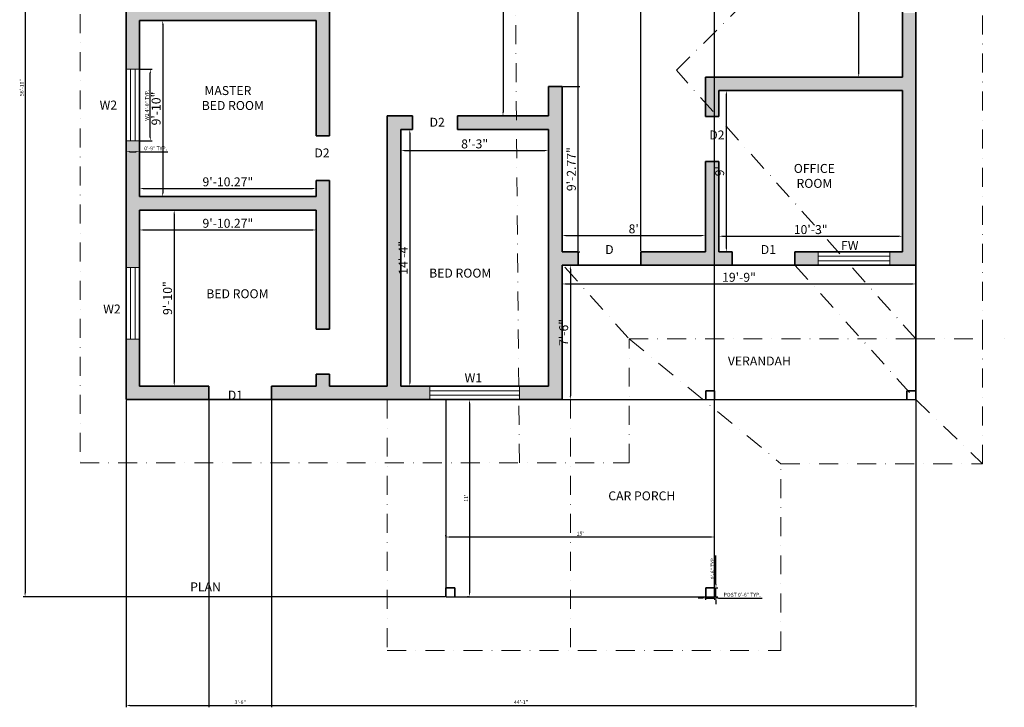
# Model space of a CAD drawing. Units: inches. Extents: x 4701 to 5398, y 2331 to 3130.
# Tile 1 of 3: x 4701 to 5360, y 2331 to 2792. Entities that reach past the tile are written whole.
import ezdxf

# ---------------------------------------------------------------- set-up
doc = ezdxf.new("R2010")
doc.units = ezdxf.units.IN
doc.linetypes.add('DASHDOT', pattern=[25.4, 12.7, -6.35, 0, -6.35])
for name, color, linetype, lineweight, true_color in [('A-ANNO-DIMS', 217, 'Continuous', 18, 0x93278f), ('A-GLAZ', 41, 'Continuous', 18, 0xf4ee51), ('A-WALL-PATT', 143, 'Continuous', 13, 0x7aafdf)]:
    doc.layers.add(name, color=color, linetype=linetype, lineweight=lineweight, true_color=true_color)
for name, color, linetype, lineweight in [('A-ANNO-TEXT', 7, 'Continuous', 18), ('A-AREA-IDEN', 7, 'Continuous', 25), ('A-COLS', 7, 'Continuous', 35), ('A-FLOR-OTLN', 7, 'Continuous', 25), ('A-ROOF-OVHD', 8, 'DASHDOT', 13), ('A-WALL', 7, 'Continuous', 35)]:
    doc.layers.add(name, color=color, linetype=linetype, lineweight=lineweight)
doc.styles.get("Standard").update_dxf_attribs({"font": 'arial.ttf'})
doc.dimstyles.new('ISO-25', dxfattribs={"dimtxt": 2.5, "dimasz": 2.5, "dimexe": 1.25, "dimexo": 0.625, "dimtad": 1, "dimlunit": 3, "dimtxsty": 'Standard', "dimcen": 2.5, "dimadec": 0, "dimazin": 0, "dimtfac": 1, "dimtmove": 0, "dimatfit": 3, "dimfxl": 1, "dimarcsym": 0})

# ---------------------------------------------------------------- blocks, each defined once
blk = doc.blocks.new('*D12')
at = {"layer": 'A-ANNO-DIMS', "color": 0, "lineweight": -2, "transparency": 16777216}
for p, q in [((5262.75, 2882.55), (5262.75, 2755.55)), ((5263.38, 2885.05), (5264, 2885.05)), ((5263.38, 2753.05), (5264, 2753.05))]:
    blk.add_line(p, q, dxfattribs=at)
at = {"layer": 'A-ANNO-DIMS', "color": 0, "transparency": 16777216}
for points in [[(5262.34, 2882.55), (5263.17, 2882.55), (5262.75, 2885.05)], [(5262.34, 2755.55), (5263.17, 2755.55), (5262.75, 2753.05)]]:
    blk.add_solid(points, dxfattribs=at)
at = {"layer": 'Defpoints', "color": 0, "transparency": 16777216}
for p in [(5262.75, 2885.05), (5262.75, 2753.05), (5262.75, 2753.05)]:
    blk.add_point(p, dxfattribs=at)
at = {"layer": 'A-ANNO-DIMS', "color": 0, "transparency": 16777216, "insert": (5259.12, 2819.05), "char_height": 6, "attachment_point": 5, "rotation": 90}
blk.add_mtext("11'", dxfattribs=at)
blk = doc.blocks.new('*D15')
at = {"layer": 'A-ANNO-DIMS', "color": 0, "lineweight": -2, "transparency": 16777216}
for p, q in [((4797.37, 2791.05), (4798, 2791.05)), ((4796.75, 2788.55), (4796.75, 2675.55)), ((4797.37, 2673.05), (4798, 2673.05))]:
    blk.add_line(p, q, dxfattribs=at)
at = {"layer": 'A-ANNO-DIMS', "color": 0, "transparency": 16777216}
for points in [[(4796.33, 2788.55), (4797.17, 2788.55), (4796.75, 2791.05)], [(4796.33, 2675.55), (4797.17, 2675.55), (4796.75, 2673.05)]]:
    blk.add_solid(points, dxfattribs=at)
at = {"layer": 'Defpoints', "color": 0, "transparency": 16777216}
for p in [(4796.75, 2791.05), (4796.75, 2673.05), (4796.75, 2673.05)]:
    blk.add_point(p, dxfattribs=at)
at = {"layer": 'A-ANNO-DIMS', "color": 0, "transparency": 16777216, "insert": (4793.06, 2732.05), "char_height": 6, "attachment_point": 5, "rotation": 90}
blk.add_mtext('9\'-10"', dxfattribs=at)
blk = doc.blocks.new('*D16')
at = {"layer": 'A-ANNO-DIMS', "color": 0, "lineweight": -2, "transparency": 16777216}
for p, q in [((4781.22, 2679.07), (4781.22, 2679.7)), ((4783.72, 2678.45), (4897, 2678.45)), ((4899.5, 2679.07), (4899.5, 2679.7))]:
    blk.add_line(p, q, dxfattribs=at)
at = {"layer": 'A-ANNO-DIMS', "color": 0, "transparency": 16777216}
for points in [[(4783.72, 2678.87), (4783.72, 2678.03), (4781.22, 2678.45)], [(4897, 2678.87), (4897, 2678.03), (4899.5, 2678.45)]]:
    blk.add_solid(points, dxfattribs=at)
at = {"layer": 'Defpoints', "color": 0, "transparency": 16777216}
for p in [(4781.22, 2678.45), (4899.5, 2678.45), (4899.5, 2678.45)]:
    blk.add_point(p, dxfattribs=at)
at = {"layer": 'A-ANNO-DIMS', "color": 0, "transparency": 16777216, "insert": (4840.36, 2682.14), "char_height": 6, "attachment_point": 5}
blk.add_mtext('9\'-10.27"', dxfattribs=at)
blk = doc.blocks.new('*D17')
at = {"layer": 'A-ANNO-DIMS', "color": 0, "lineweight": -2, "transparency": 16777216}
for p, q in [((4805.06, 2664.05), (4805.69, 2664.05)), ((4804.44, 2661.55), (4804.44, 2548.55)), ((4805.06, 2546.05), (4805.69, 2546.05))]:
    blk.add_line(p, q, dxfattribs=at)
at = {"layer": 'A-ANNO-DIMS', "color": 0, "transparency": 16777216}
for points in [[(4804.02, 2661.55), (4804.86, 2661.55), (4804.44, 2664.05)], [(4804.02, 2548.55), (4804.86, 2548.55), (4804.44, 2546.05)]]:
    blk.add_solid(points, dxfattribs=at)
at = {"layer": 'Defpoints', "color": 0, "transparency": 16777216}
for p in [(4804.44, 2664.05), (4804.44, 2546.05), (4804.44, 2546.05)]:
    blk.add_point(p, dxfattribs=at)
at = {"layer": 'A-ANNO-DIMS', "color": 0, "transparency": 16777216, "insert": (4800.75, 2605.05), "char_height": 6, "attachment_point": 5, "rotation": 90}
blk.add_mtext('9\'-10"', dxfattribs=at)
blk = doc.blocks.new('*D18')
at = {"layer": 'A-ANNO-DIMS', "color": 0, "lineweight": -2, "transparency": 16777216}
for p, q in [((4781.22, 2651.33), (4781.22, 2651.95)), ((4783.72, 2650.7), (4897, 2650.7)), ((4899.5, 2651.33), (4899.5, 2651.95))]:
    blk.add_line(p, q, dxfattribs=at)
at = {"layer": 'A-ANNO-DIMS', "color": 0, "transparency": 16777216}
for points in [[(4783.72, 2651.12), (4783.72, 2650.29), (4781.22, 2650.7)], [(4897, 2651.12), (4897, 2650.29), (4899.5, 2650.7)]]:
    blk.add_solid(points, dxfattribs=at)
at = {"layer": 'Defpoints', "color": 0, "transparency": 16777216}
for p in [(4781.22, 2650.7), (4899.5, 2650.7), (4899.5, 2650.7)]:
    blk.add_point(p, dxfattribs=at)
at = {"layer": 'A-ANNO-DIMS', "color": 0, "transparency": 16777216, "insert": (4840.36, 2654.39), "char_height": 6, "attachment_point": 5}
blk.add_mtext('9\'-10.27"', dxfattribs=at)
blk = doc.blocks.new('*D19')
at = {"layer": 'A-ANNO-DIMS', "color": 0, "lineweight": -2, "transparency": 16777216}
for p, q in [((4961.57, 2718.05), (4960.94, 2718.05)), ((4962.19, 2715.55), (4962.19, 2548.55)), ((4961.57, 2546.05), (4960.94, 2546.05))]:
    blk.add_line(p, q, dxfattribs=at)
at = {"layer": 'A-ANNO-DIMS', "color": 0, "transparency": 16777216}
for points in [[(4961.78, 2715.55), (4962.61, 2715.55), (4962.19, 2718.05)], [(4961.78, 2548.55), (4962.61, 2548.55), (4962.19, 2546.05)]]:
    blk.add_solid(points, dxfattribs=at)
at = {"layer": 'Defpoints', "color": 0, "transparency": 16777216}
for p in [(4962.19, 2718.05), (4962.19, 2546.05), (4962.19, 2546.05)]:
    blk.add_point(p, dxfattribs=at)
at = {"layer": 'A-ANNO-DIMS', "color": 0, "transparency": 16777216, "insert": (4958.56, 2632.05), "char_height": 6, "attachment_point": 5, "rotation": 90}
blk.add_mtext('14\'-4"', dxfattribs=at)
blk = doc.blocks.new('*D20')
at = {"layer": 'A-ANNO-DIMS', "color": 0, "lineweight": -2, "transparency": 16777216}
for p, q in [((4956.11, 2704.5), (4956.11, 2705.12)), ((4958.61, 2703.87), (5052.61, 2703.87)), ((5055.11, 2704.5), (5055.11, 2705.12))]:
    blk.add_line(p, q, dxfattribs=at)
at = {"layer": 'A-ANNO-DIMS', "color": 0, "transparency": 16777216}
for points in [[(4958.61, 2704.29), (4958.61, 2703.46), (4956.11, 2703.87)], [(5052.61, 2704.29), (5052.61, 2703.46), (5055.11, 2703.87)]]:
    blk.add_solid(points, dxfattribs=at)
at = {"layer": 'Defpoints', "color": 0, "transparency": 16777216}
for p in [(4956.11, 2703.87), (5055.11, 2703.87), (5055.11, 2703.87)]:
    blk.add_point(p, dxfattribs=at)
at = {"layer": 'A-ANNO-DIMS', "color": 0, "transparency": 16777216, "insert": (5005.61, 2707.56), "char_height": 6, "attachment_point": 5}
blk.add_mtext('8\'-3"', dxfattribs=at)
blk = doc.blocks.new('*D21')
at = {"layer": 'A-ANNO-DIMS', "color": 0, "lineweight": -2, "transparency": 16777216}
for p, q in [((5001.51, 2537.05), (5000.88, 2537.05)), ((5002.13, 2534.55), (5002.13, 2407.55)), ((5001.51, 2405.05), (5000.88, 2405.05))]:
    blk.add_line(p, q, dxfattribs=at)
at = {"layer": 'A-ANNO-DIMS', "color": 0, "transparency": 16777216}
for points in [[(5001.72, 2534.55), (5002.55, 2534.55), (5002.13, 2537.05)], [(5001.72, 2407.55), (5002.55, 2407.55), (5002.13, 2405.05)]]:
    blk.add_solid(points, dxfattribs=at)
at = {"layer": 'Defpoints', "color": 0, "transparency": 16777216}
for p in [(5002.13, 2537.05), (5002.13, 2405.05), (5002.13, 2405.05)]:
    blk.add_point(p, dxfattribs=at)
at = {"layer": 'A-ANNO-DIMS', "color": 0, "transparency": 16777216, "insert": (5000.25, 2471.05), "char_height": 2.5, "attachment_point": 5, "rotation": 90}
blk.add_mtext("11'", dxfattribs=at)
blk = doc.blocks.new('*D22')
at = {"layer": 'A-ANNO-DIMS', "color": 0, "lineweight": -2, "transparency": 16777216}
for p, q in [((4986.3, 2445.66), (4986.3, 2446.29)), ((5166.3, 2445.66), (5166.3, 2446.29)), ((4988.8, 2445.04), (5163.8, 2445.04))]:
    blk.add_line(p, q, dxfattribs=at)
at = {"layer": 'A-ANNO-DIMS', "color": 0, "transparency": 16777216}
for points in [[(4988.8, 2445.45), (4988.8, 2444.62), (4986.3, 2445.04)], [(5163.8, 2445.45), (5163.8, 2444.62), (5166.3, 2445.04)]]:
    blk.add_solid(points, dxfattribs=at)
at = {"layer": 'Defpoints', "color": 0, "transparency": 16777216}
for p in [(4986.3, 2445.04), (5166.3, 2445.04), (5166.3, 2445.04)]:
    blk.add_point(p, dxfattribs=at)
at = {"layer": 'A-ANNO-DIMS', "color": 0, "transparency": 16777216, "insert": (5076.3, 2446.94), "char_height": 2.5, "attachment_point": 5}
blk.add_mtext("15'", dxfattribs=at)
blk = doc.blocks.new('*D23')
at = {"layer": 'A-ANNO-DIMS', "color": 0, "lineweight": -2, "transparency": 16777216}
for p, q in [((5064.11, 2615.15), (5064.11, 2615.78)), ((5066.61, 2614.53), (5298.61, 2614.53)), ((5301.11, 2615.15), (5301.11, 2615.78))]:
    blk.add_line(p, q, dxfattribs=at)
at = {"layer": 'A-ANNO-DIMS', "color": 0, "transparency": 16777216}
for points in [[(5066.61, 2614.94), (5066.61, 2614.11), (5064.11, 2614.53)], [(5298.61, 2614.94), (5298.61, 2614.11), (5301.11, 2614.53)]]:
    blk.add_solid(points, dxfattribs=at)
at = {"layer": 'Defpoints', "color": 0, "transparency": 16777216}
for p in [(5064.11, 2614.53), (5301.11, 2614.53), (5301.11, 2614.53)]:
    blk.add_point(p, dxfattribs=at)
at = {"layer": 'A-ANNO-DIMS', "color": 0, "transparency": 16777216, "insert": (5182.61, 2618.22), "char_height": 6, "attachment_point": 5}
blk.add_mtext('19\'-9"', dxfattribs=at)
blk = doc.blocks.new('*D24')
at = {"layer": 'A-ANNO-DIMS', "color": 0, "lineweight": -2, "transparency": 16777216}
for p, q in [((5069.69, 2624.55), (5069.69, 2539.55)), ((5070.31, 2627.05), (5070.94, 2627.05)), ((5070.31, 2537.05), (5070.94, 2537.05))]:
    blk.add_line(p, q, dxfattribs=at)
at = {"layer": 'A-ANNO-DIMS', "color": 0, "transparency": 16777216}
for points in [[(5069.27, 2624.55), (5070.1, 2624.55), (5069.69, 2627.05)], [(5069.27, 2539.55), (5070.1, 2539.55), (5069.69, 2537.05)]]:
    blk.add_solid(points, dxfattribs=at)
at = {"layer": 'Defpoints', "color": 0, "transparency": 16777216}
for p in [(5069.69, 2627.05), (5069.69, 2537.05), (5069.69, 2537.05)]:
    blk.add_point(p, dxfattribs=at)
at = {"layer": 'A-ANNO-DIMS', "color": 0, "transparency": 16777216, "insert": (5066, 2582.05), "char_height": 6, "attachment_point": 5, "rotation": 90}
blk.add_mtext('7\'-6"', dxfattribs=at)
blk = doc.blocks.new('*D25')
at = {"layer": 'A-ANNO-DIMS', "color": 0, "lineweight": -2, "transparency": 16777216}
for p, q in [((5064.11, 2647.58), (5064.11, 2648.21)), ((5066.61, 2646.96), (5157.61, 2646.96)), ((5160.11, 2647.58), (5160.11, 2648.21))]:
    blk.add_line(p, q, dxfattribs=at)
at = {"layer": 'A-ANNO-DIMS', "color": 0, "transparency": 16777216}
for points in [[(5066.61, 2647.38), (5066.61, 2646.54), (5064.11, 2646.96)], [(5157.61, 2647.38), (5157.61, 2646.54), (5160.11, 2646.96)]]:
    blk.add_solid(points, dxfattribs=at)
at = {"layer": 'Defpoints', "color": 0, "transparency": 16777216}
for p in [(5064.11, 2646.96), (5160.11, 2646.96), (5160.11, 2646.96)]:
    blk.add_point(p, dxfattribs=at)
at = {"layer": 'A-ANNO-DIMS', "color": 0, "transparency": 16777216, "insert": (5112.11, 2650.65), "char_height": 6, "attachment_point": 5}
blk.add_mtext("8'", dxfattribs=at)
blk = doc.blocks.new('*D26')
at = {"layer": 'A-ANNO-DIMS', "color": 0, "lineweight": -2, "transparency": 16777216}
for p, q in [((5064.73, 2746.83), (5076.07, 2746.83)), ((5074.82, 2638.55), (5074.82, 2744.33)), ((5070.84, 2636.05), (5076.07, 2636.05))]:
    blk.add_line(p, q, dxfattribs=at)
at = {"layer": 'A-ANNO-DIMS', "color": 0, "transparency": 16777216}
for points in [[(5074.4, 2744.33), (5075.24, 2744.33), (5074.82, 2746.83)], [(5074.4, 2638.55), (5075.24, 2638.55), (5074.82, 2636.05)]]:
    blk.add_solid(points, dxfattribs=at)
at = {"layer": 'Defpoints', "color": 0, "transparency": 16777216}
for p in [(5064.11, 2746.83), (5074.82, 2746.83), (5070.21, 2636.05)]:
    blk.add_point(p, dxfattribs=at)
at = {"layer": 'A-ANNO-DIMS', "color": 0, "transparency": 16777216, "insert": (5071.13, 2691.44), "char_height": 6, "attachment_point": 5, "rotation": 90}
blk.add_mtext('9\'-2.77"', dxfattribs=at)
blk = doc.blocks.new('*D27')
at = {"layer": 'A-ANNO-DIMS', "color": 0, "lineweight": -2, "transparency": 16777216}
for p, q in [((5169.11, 2647.11), (5169.11, 2647.74)), ((5171.61, 2646.49), (5289.61, 2646.49)), ((5292.11, 2647.11), (5292.11, 2647.74))]:
    blk.add_line(p, q, dxfattribs=at)
at = {"layer": 'A-ANNO-DIMS', "color": 0, "transparency": 16777216}
for points in [[(5171.61, 2646.9), (5171.61, 2646.07), (5169.11, 2646.49)], [(5289.61, 2646.9), (5289.61, 2646.07), (5292.11, 2646.49)]]:
    blk.add_solid(points, dxfattribs=at)
at = {"layer": 'Defpoints', "color": 0, "transparency": 16777216}
for p in [(5169.11, 2646.49), (5292.11, 2646.49), (5292.11, 2646.49)]:
    blk.add_point(p, dxfattribs=at)
at = {"layer": 'A-ANNO-DIMS', "color": 0, "transparency": 16777216, "insert": (5230.61, 2650.18), "char_height": 6, "attachment_point": 5}
blk.add_mtext('10\'-3"', dxfattribs=at)
blk = doc.blocks.new('*D28')
at = {"layer": 'A-ANNO-DIMS', "color": 0, "lineweight": -2, "transparency": 16777216}
for p, q in [((5174.78, 2744.05), (5175.4, 2744.05)), ((5174.15, 2638.55), (5174.15, 2741.55)), ((5174.78, 2636.05), (5175.4, 2636.05))]:
    blk.add_line(p, q, dxfattribs=at)
at = {"layer": 'A-ANNO-DIMS', "color": 0, "transparency": 16777216}
for points in [[(5173.74, 2741.55), (5174.57, 2741.55), (5174.15, 2744.05)], [(5173.74, 2638.55), (5174.57, 2638.55), (5174.15, 2636.05)]]:
    blk.add_solid(points, dxfattribs=at)
at = {"layer": 'Defpoints', "color": 0, "transparency": 16777216}
for p in [(5174.15, 2744.05), (5174.15, 2744.05), (5174.15, 2636.05)]:
    blk.add_point(p, dxfattribs=at)
at = {"layer": 'A-ANNO-DIMS', "color": 0, "transparency": 16777216, "insert": (5170.46, 2690.05), "char_height": 6, "attachment_point": 5, "rotation": 90}
blk.add_mtext("9'", dxfattribs=at)
blk = doc.blocks.new('*D30')
at = {"layer": 'A-ANNO-DIMS', "color": 0, "lineweight": -2, "transparency": 16777216}
for p, q in [((5024.48, 2894.05), (5023.35, 2894.05)), ((5024.6, 2891.55), (5024.6, 2729.55)), ((5025.23, 2727.05), (5025.85, 2727.05))]:
    blk.add_line(p, q, dxfattribs=at)
at = {"layer": 'A-ANNO-DIMS', "color": 0, "transparency": 16777216}
for points in [[(5024.19, 2891.55), (5025.02, 2891.55), (5024.6, 2894.05)], [(5024.19, 2729.55), (5025.02, 2729.55), (5024.6, 2727.05)]]:
    blk.add_solid(points, dxfattribs=at)
at = {"layer": 'Defpoints', "color": 0, "transparency": 16777216}
for p in [(5025.11, 2894.05), (5024.6, 2727.05), (5024.6, 2727.05)]:
    blk.add_point(p, dxfattribs=at)
at = {"layer": 'A-ANNO-DIMS', "color": 0, "transparency": 16777216, "insert": (5022.7, 2810.55), "char_height": 2.5, "attachment_point": 5, "rotation": 90}
blk.add_mtext('13\'-11"', dxfattribs=at)
blk = doc.blocks.new('WIN-48IN')
for p, q in [((0, 48), (9, 48)), ((0, 48), (0, 0)), ((3, 48), (3, 0)), ((6, 48), (6, 0)), ((9, 0), (9, 48)), ((0, 0), (9, 0))]:
    blk.add_line(p, q)
blk = doc.blocks.new('WIN-60IN')
for p, q in [((0, 9), (0, 0)), ((0, 9), (60, 9)), ((60, 9), (60, 0)), ((0, 6), (60, 6)), ((0, 3), (60, 3)), ((60, 0), (0, 0))]:
    blk.add_line(p, q)
blk = doc.blocks.new('POST-6X6IN')
for p, q in [((0, 0), (0, 6)), ((0, 6), (6, 6)), ((6, 6), (6, 0))]:
    blk.add_line(p, q)
blk = doc.blocks.new('*D35')
at = {"layer": 'A-ANNO-DIMS', "color": 0, "lineweight": -2, "transparency": 16777216}
for p, q in [((4781.85, 2758.33), (4789.67, 2758.33)), ((4788.42, 2712.83), (4788.42, 2755.83)), ((4781.85, 2710.33), (4789.67, 2710.33))]:
    blk.add_line(p, q, dxfattribs=at)
at = {"layer": 'A-ANNO-DIMS', "color": 0, "transparency": 16777216}
for points in [[(4788.01, 2755.83), (4788.84, 2755.83), (4788.42, 2758.33)], [(4788.01, 2712.83), (4788.84, 2712.83), (4788.42, 2710.33)]]:
    blk.add_solid(points, dxfattribs=at)
at = {"layer": 'Defpoints', "color": 0, "transparency": 16777216}
for p in [(4781.22, 2758.33), (4788.42, 2758.33), (4781.22, 2710.33)]:
    blk.add_point(p, dxfattribs=at)
at = {"layer": 'A-ANNO-DIMS', "color": 0, "transparency": 16777216, "insert": (4786.52, 2734.33), "char_height": 2.5, "attachment_point": 5, "rotation": 90}
blk.add_mtext('W2 4\'-0" TYP.', dxfattribs=at)
blk = doc.blocks.new('*D36')
at = {"layer": 'A-ANNO-DIMS', "color": 0, "lineweight": -2, "transparency": 16777216}
for p, q in [((4772.22, 2709.71), (4772.22, 2701.88)), ((4781.22, 2709.71), (4781.22, 2701.88)), ((4774.72, 2703.13), (4778.72, 2703.13)), ((4781.22, 2703.13), (4800.21, 2703.13))]:
    blk.add_line(p, q, dxfattribs=at)
at = {"layer": 'A-ANNO-DIMS', "color": 0, "transparency": 16777216}
for points in [[(4774.72, 2703.55), (4774.72, 2702.72), (4772.22, 2703.13)], [(4778.72, 2703.55), (4778.72, 2702.72), (4781.22, 2703.13)]]:
    blk.add_solid(points, dxfattribs=at)
at = {"layer": 'Defpoints', "color": 0, "transparency": 16777216}
for p in [(4772.22, 2710.33), (4781.22, 2710.33), (4781.22, 2703.13)]:
    blk.add_point(p, dxfattribs=at)
at = {"layer": 'A-ANNO-DIMS', "color": 0, "transparency": 16777216, "insert": (4791.97, 2705.04), "char_height": 2.5, "attachment_point": 5}
blk.add_mtext('0\'-9" TYP.', dxfattribs=at)
blk = doc.blocks.new('*D41')
at = {"layer": 'A-ANNO-DIMS', "color": 0, "lineweight": -2, "transparency": 16777216}
for p, q in [((5157.8, 2404.15), (5155.3, 2404.15)), ((5160.3, 2404.43), (5160.3, 2402.9)), ((5160.3, 2404.15), (5166.3, 2404.15)), ((5166.3, 2404.43), (5166.3, 2402.9)), ((5168.8, 2404.15), (5198.15, 2404.15))]:
    blk.add_line(p, q, dxfattribs=at)
at = {"layer": 'A-ANNO-DIMS', "color": 0, "transparency": 16777216}
for points in [[(5157.8, 2404.57), (5157.8, 2403.74), (5160.3, 2404.15)], [(5168.8, 2404.57), (5168.8, 2403.74), (5166.3, 2404.15)]]:
    blk.add_solid(points, dxfattribs=at)
at = {"layer": 'Defpoints', "color": 0, "transparency": 16777216}
for p in [(5160.3, 2405.05), (5166.3, 2405.05), (5166.3, 2404.15)]:
    blk.add_point(p, dxfattribs=at)
at = {"layer": 'A-ANNO-DIMS', "color": 0, "transparency": 16777216, "insert": (5184.73, 2406.07), "char_height": 2.5, "attachment_point": 5}
blk.add_mtext('POST 0\'-6" TYP.', dxfattribs=at)
blk = doc.blocks.new('*D42')
at = {"layer": 'A-ANNO-DIMS', "color": 0, "lineweight": -2, "transparency": 16777216}
for p, q in [((5167.2, 2413.55), (5167.2, 2432.54)), ((5166.93, 2411.05), (5168.45, 2411.05)), ((5167.2, 2405.05), (5167.2, 2411.05)), ((5166.93, 2405.05), (5168.45, 2405.05)), ((5167.2, 2402.55), (5167.2, 2400.05))]:
    blk.add_line(p, q, dxfattribs=at)
at = {"layer": 'A-ANNO-DIMS', "color": 0, "transparency": 16777216}
for points in [[(5166.79, 2413.55), (5167.62, 2413.55), (5167.2, 2411.05)], [(5166.79, 2402.55), (5167.62, 2402.55), (5167.2, 2405.05)]]:
    blk.add_solid(points, dxfattribs=at)
at = {"layer": 'Defpoints', "color": 0, "transparency": 16777216}
for p in [(5166.3, 2411.05), (5167.2, 2411.05), (5166.3, 2405.05)]:
    blk.add_point(p, dxfattribs=at)
at = {"layer": 'A-ANNO-DIMS', "color": 0, "transparency": 16777216, "insert": (5165.3, 2424.3), "char_height": 2.5, "attachment_point": 5, "rotation": 90}
blk.add_mtext('0\'-6" TYP.', dxfattribs=at)
blk = doc.blocks.new('*D43')
at = {"layer": 'A-ANNO-DIMS', "color": 0, "lineweight": -2, "transparency": 16777216}
for p, q in [((4772.22, 2536.43), (4772.22, 2330.95)), ((5301.11, 2536.43), (5301.11, 2330.95)), ((4774.72, 2332.2), (5298.61, 2332.2))]:
    blk.add_line(p, q, dxfattribs=at)
at = {"layer": 'A-ANNO-DIMS', "color": 0, "transparency": 16777216}
for points in [[(4774.72, 2332.62), (4774.72, 2331.79), (4772.22, 2332.2)], [(5298.61, 2332.62), (5298.61, 2331.79), (5301.11, 2332.2)]]:
    blk.add_solid(points, dxfattribs=at)
at = {"layer": 'Defpoints', "color": 0, "transparency": 16777216}
for p in [(4772.22, 2537.05), (5301.11, 2537.05), (5301.11, 2332.2)]:
    blk.add_point(p, dxfattribs=at)
at = {"layer": 'A-ANNO-DIMS', "color": 0, "transparency": 16777216, "insert": (5036.67, 2334.08), "char_height": 2.5, "attachment_point": 5}
blk.add_mtext('44\'-1"', dxfattribs=at)
blk = doc.blocks.new('*D44')
at = {"layer": 'A-ANNO-DIMS', "color": 0, "lineweight": -2, "transparency": 16777216}
for p, q in [((4863.6, 3087.05), (4703.32, 3087.05)), ((4704.57, 3084.55), (4704.57, 2407.55)), ((4985.68, 2405.05), (4703.32, 2405.05))]:
    blk.add_line(p, q, dxfattribs=at)
at = {"layer": 'A-ANNO-DIMS', "color": 0, "transparency": 16777216}
for points in [[(4704.15, 3084.55), (4704.99, 3084.55), (4704.57, 3087.05)], [(4704.15, 2407.55), (4704.99, 2407.55), (4704.57, 2405.05)]]:
    blk.add_solid(points, dxfattribs=at)
at = {"layer": 'Defpoints', "color": 0, "transparency": 16777216}
for p in [(4864.22, 3087.05), (4704.57, 2405.05), (4986.3, 2405.05)]:
    blk.add_point(p, dxfattribs=at)
at = {"layer": 'A-ANNO-DIMS', "color": 0, "transparency": 16777216, "insert": (4702.67, 2746.05), "char_height": 2.5, "attachment_point": 5, "rotation": 90}
blk.add_mtext('56\'-10"', dxfattribs=at)
blk = doc.blocks.new('*D45')
at = {"layer": 'A-ANNO-DIMS', "color": 0, "lineweight": -2, "transparency": 16777216}
for p, q in [((4827.66, 2536.43), (4827.66, 2330.95)), ((4869.66, 2536.43), (4869.66, 2330.95)), ((4830.16, 2332.2), (4867.16, 2332.2))]:
    blk.add_line(p, q, dxfattribs=at)
at = {"layer": 'A-ANNO-DIMS', "color": 0, "transparency": 16777216}
for points in [[(4830.16, 2332.62), (4830.16, 2331.79), (4827.66, 2332.2)], [(4867.16, 2332.62), (4867.16, 2331.79), (4869.66, 2332.2)]]:
    blk.add_solid(points, dxfattribs=at)
at = {"layer": 'Defpoints', "color": 0, "transparency": 16777216}
for p in [(4827.66, 2537.05), (4869.66, 2537.05), (4869.66, 2332.2)]:
    blk.add_point(p, dxfattribs=at)
at = {"layer": 'A-ANNO-DIMS', "color": 0, "transparency": 16777216, "insert": (4848.66, 2334.11), "char_height": 2.5, "attachment_point": 5}
blk.add_mtext('3\'-6"', dxfattribs=at)
blk = doc.blocks.new('*D48')
at = {"layer": 'A-ANNO-DIMS', "color": 0, "lineweight": -2, "transparency": 16777216}
for p, q in [((5074.82, 2636.68), (5074.82, 3125.15)), ((5116.82, 2636.68), (5116.82, 3125.15)), ((5077.32, 3123.9), (5114.32, 3123.9))]:
    blk.add_line(p, q, dxfattribs=at)
at = {"layer": 'A-ANNO-DIMS', "color": 0, "transparency": 16777216}
for points in [[(5077.32, 3124.32), (5077.32, 3123.49), (5074.82, 3123.9)], [(5114.32, 3124.32), (5114.32, 3123.49), (5116.82, 3123.9)]]:
    blk.add_solid(points, dxfattribs=at)
at = {"layer": 'Defpoints', "color": 0, "transparency": 16777216}
for p in [(5116.82, 3123.9), (5074.82, 2636.05), (5116.82, 2636.05)]:
    blk.add_point(p, dxfattribs=at)
at = {"layer": 'A-ANNO-DIMS', "color": 0, "transparency": 16777216, "insert": (5095.82, 3125.81), "char_height": 2.5, "attachment_point": 5}
blk.add_mtext('3\'-6"', dxfattribs=at)
blk = doc.blocks.new('*D50')
at = {"layer": 'A-ANNO-DIMS', "color": 0, "lineweight": -2, "transparency": 16777216}
for p, q in [((5166.3, 2537.68), (5166.3, 3125.15)), ((5301.11, 2537.68), (5301.11, 3125.15)), ((5168.8, 3123.9), (5298.61, 3123.9))]:
    blk.add_line(p, q, dxfattribs=at)
at = {"layer": 'A-ANNO-DIMS', "color": 0, "transparency": 16777216}
for points in [[(5168.8, 3124.32), (5168.8, 3123.49), (5166.3, 3123.9)], [(5298.61, 3124.32), (5298.61, 3123.49), (5301.11, 3123.9)]]:
    blk.add_solid(points, dxfattribs=at)
at = {"layer": 'Defpoints', "color": 0, "transparency": 16777216}
for p in [(5301.11, 3123.9), (5166.3, 2537.05), (5301.11, 2537.05)]:
    blk.add_point(p, dxfattribs=at)
at = {"layer": 'A-ANNO-DIMS', "color": 0, "transparency": 16777216, "insert": (5233.71, 3125.81), "char_height": 2.5, "attachment_point": 5}
blk.add_mtext('11\'-3"', dxfattribs=at)

msp = doc.modelspace()

# ---------------------------------------------------------------- hatches: boundary and pattern name
at = {"layer": 'A-WALL-PATT'}
h = msp.add_hatch(color=256, dxfattribs=at)
h.dxf.hatch_style = 1
h.paths.add_polyline_path([(4829.723, 3062.054), (4820.723, 3062.054), (4772.223, 3062.054), (4772.223, 3050.208), (4781.223, 3050.208), (4781.223, 3053.054), (4820.723, 3053.054), (4820.723, 3050.208), (4829.723, 3050.208)])
h.paths.add_polyline_path([(4781.223, 3050.208), (4772.223, 3050.208), (4772.223, 3029.054), (4772.223, 2999.675), (4781.223, 2999.675), (4781.223, 3029.054)])
h.paths.add_polyline_path([(4781.223, 2918.054), (4864.223, 2918.054), (4899.497, 2918.054), (4899.497, 2845.832), (4908.497, 2845.832), (4908.497, 2918.054), (4908.497, 2927.054), (4893.11, 2927.054), (4893.11, 2954.328), (4884.11, 2954.328), (4884.11, 2927.054), (4864.223, 2927.054), (4781.223, 2927.054), (4781.223, 2951.675), (4772.223, 2951.675), (4772.223, 2918.054), (4772.223, 2884.79), (4781.223, 2884.79)])
h.paths.add_polyline_path([(4893.11, 3029.054), (4908.497, 3029.054), (4908.497, 3038.054), (4873.223, 3038.054), (4873.223, 3050.208), (4864.223, 3050.208), (4864.223, 3038.054), (4859.723, 3038.054), (4859.723, 3029.054), (4884.11, 3029.054), (4884.11, 2984.328), (4893.11, 2984.328)])
h.paths.add_polyline_path([(4873.223, 3078.054), (4878.497, 3078.054), (4878.497, 3087.054), (4864.223, 3087.054), (4864.223, 3050.208), (4873.223, 3050.208)])
h.paths.add_polyline_path([(4976.546, 3087.054), (4908.497, 3087.054), (4908.497, 3078.054), (4944.223, 3078.054), (4944.223, 3056.054), (4953.223, 3056.054), (4953.223, 3078.054), (4976.546, 3078.054)])
h.paths.add_polyline_path([(5044.223, 3087.054), (5000.546, 3087.054), (5000.546, 3078.054), (5035.223, 3078.054), (5035.223, 3038.054), (5044.223, 3038.054)])
h.paths.add_polyline_path([(5030.994, 3038.054), (5017.16, 3038.054), (4944.223, 3038.054), (4944.223, 3029.054), (5031.069, 3029.054)])
h.paths.add_polyline_path([(5044.223, 3038.054), (5035.223, 3038.054), (5030.994, 3038.054), (5031.069, 3029.054), (5044.223, 3029.054)])
h.paths.add_polyline_path([(5202.11, 3005.054), (5193.11, 3005.054), (5031.27, 3005.054), (5031.345, 2996.054), (5193.11, 2996.054), (5193.11, 2978.066), (5202.11, 2978.066), (5202.11, 2996.054)])
h.paths.add_polyline_path([(5031.27, 3005.054), (5025.11, 3005.054), (5016.11, 3005.054), (5016.11, 2903.054), (4962.304, 2903.054), (4962.304, 2894.054), (5025.11, 2894.054), (5025.11, 2996.054), (5031.345, 2996.054)])
h.paths.add_polyline_path([(5278.045, 2894.054), (5202.11, 2894.054), (5202.11, 2900.054), (5202.11, 2918.066), (5193.11, 2918.066), (5193.11, 2900.054), (5193.11, 2894.054), (5055.11, 2894.054), (5055.11, 2840.014), (5055.11, 2813.236), (5064.11, 2813.236), (5064.11, 2840.014), (5064.11, 2885.054), (5268.987, 2885.054)])
h.paths.add_polyline_path([(5301.11, 2894.054), (5278.045, 2894.054), (5268.987, 2885.054), (5292.11, 2885.054), (5292.11, 2855.934), (5301.11, 2855.934), (5301.11, 2885.054)])
h.paths.add_polyline_path([(5301.11, 2795.934), (5292.11, 2795.934), (5292.11, 2753.054), (5193.11, 2753.054), (5160.11, 2753.054), (5160.11, 2735.907), (5168.378, 2726.63), (5169.11, 2726.63), (5169.11, 2744.054), (5292.11, 2744.054), (5292.11, 2636.054), (5283.654, 2636.054), (5283.654, 2627.054), (5301.11, 2627.054)])
h.paths.add_polyline_path([(5160.11, 2735.907), (5160.11, 2726.63), (5168.378, 2726.63)], flags=17)
h.paths.add_polyline_path([(5064.11, 2746.827), (5055.11, 2746.827), (5055.11, 2727.054), (5033.595, 2727.054), (5033.671, 2718.054), (5055.11, 2718.054), (5055.11, 2627.054), (5055.11, 2546.054), (5035.539, 2546.054), (5035.539, 2537.054), (5064.11, 2537.054), (5064.11, 2627.054), (5074.819, 2627.054), (5074.819, 2636.054), (5064.11, 2636.054)])
h.paths.add_polyline_path([(5178.11, 2636.054), (5169.11, 2636.054), (5169.11, 2696.63), (5160.11, 2696.63), (5160.11, 2636.054), (5116.819, 2636.054), (5116.819, 2627.054), (5178.11, 2627.054)])
h.paths.add_polyline_path([(5235.654, 2636.054), (5220.11, 2636.054), (5220.11, 2627.054), (5235.654, 2627.054)], flags=17)
h.paths.add_polyline_path([(5033.595, 2727.054), (4994.096, 2727.054), (4994.096, 2718.054), (5033.671, 2718.054)])
h.paths.add_polyline_path([(4964.096, 2727.054), (4947.11, 2727.054), (4947.11, 2546.054), (4908.497, 2546.054), (4908.497, 2554.169), (4899.497, 2554.169), (4899.497, 2546.054), (4869.656, 2546.054), (4869.656, 2537.054), (4908.497, 2537.054), (4975.539, 2537.054), (4975.539, 2546.054), (4956.11, 2546.054), (4956.11, 2718.054), (4964.096, 2718.054)])
h.paths.add_polyline_path([(4827.656, 2546.054), (4781.223, 2546.054), (4781.223, 2577.475), (4772.223, 2577.475), (4772.223, 2537.054), (4827.656, 2537.054)])
h.paths.add_polyline_path([(4781.223, 2664.054), (4899.497, 2664.054), (4899.497, 2584.169), (4908.497, 2584.169), (4908.497, 2683.844), (4899.497, 2683.844), (4899.497, 2673.054), (4781.223, 2673.054), (4781.223, 2710.334), (4772.223, 2710.334), (4772.223, 2625.475), (4781.223, 2625.475)])
h.paths.add_polyline_path([(4908.497, 2815.832), (4899.497, 2815.832), (4899.497, 2800.054), (4864.223, 2800.054), (4781.223, 2800.054), (4781.223, 2836.79), (4772.223, 2836.79), (4772.223, 2758.334), (4781.223, 2758.334), (4781.223, 2791.054), (4899.497, 2791.054), (4899.497, 2713.844), (4908.497, 2713.844)])

# ---------------------------------------------------------------- linework, layer by layer
at = {"layer": 'A-FLOR-OTLN'}
for p, q in [((4986.304, 2537.054), (4986.304, 2405.054)), ((5064.11, 2537.054), (5301.11, 2537.054)), ((5166.304, 2405.054), (5166.304, 2537.054)), ((4986.304, 2405.054), (5166.304, 2405.054))]:
    msp.add_line(p, q, dxfattribs=at)
at = {"layer": 'A-ROOF-OVHD'}
for p, q in [((4741.42, 3050.208), (4741.42, 2494.747)), ((5035.539, 2494.747), (5030.892, 3050.253)), ((5140.745, 2757.635), (5308.37, 2924.185)), ((5345.573, 2577.697), (5345.573, 2924.185)), ((5301.11, 2577.697), (5140.745, 2757.635)), ((5140.745, 2757.635), (5140.745, 2757.635)), ((5065.935, 2625.804), (5109.029, 2577.697)), ((5220.11, 2627.054), (5301.11, 2537.054)), ((5109.029, 2494.747), (5109.029, 2577.697)), ((5109.029, 2577.697), (5301.11, 2577.697)), ((5109.029, 2577.697), (5210.732, 2494.147)), ((5301.11, 2577.697), (5345.573, 2577.697)), ((5345.573, 2494.147), (5345.573, 2577.697)), ((5360.274, 2577.697), (5360.274, 2577.697)), ((4947.11, 2537.054), (4947.11, 2369.054)), ((5069.685, 2537.054), (5069.685, 2369.054)), ((5301.11, 2537.054), (5345.573, 2494.147)), ((4741.42, 2494.747), (5109.029, 2494.747)), ((5210.732, 2369.054), (5210.732, 2494.147)), ((5210.732, 2494.147), (5345.573, 2494.147)), ((4947.11, 2369.054), (5210.732, 2369.054))]:
    msp.add_line(p, q, dxfattribs=at)
at = {"layer": 'A-WALL'}
for p, q in [((4772.223, 2918.054), (4772.223, 2537.054)), ((5292.11, 2840.014), (5292.11, 2753.054)), ((5292.11, 2840.014), (5292.11, 2753.054)), ((5301.11, 2840.014), (5301.11, 2537.054)), ((4908.497, 2815.832), (4908.497, 2713.844)), ((4781.223, 2791.054), (4864.223, 2791.054)), ((4781.223, 2791.054), (4899.497, 2791.054)), ((4781.223, 2791.054), (4781.223, 2673.054)), ((4899.497, 2791.054), (4864.223, 2791.054)), ((4899.497, 2791.054), (4899.497, 2713.844)), ((5160.11, 2753.054), (5193.11, 2753.054)), ((5160.11, 2753.054), (5160.11, 2726.63)), ((5292.11, 2753.054), (5193.11, 2753.054)), ((5055.11, 2746.827), (5055.11, 2727.054)), ((5055.11, 2746.827), (5064.11, 2746.827)), ((5064.11, 2746.827), (5064.11, 2636.054)), ((5169.11, 2744.054), (5292.11, 2744.054)), ((5169.11, 2744.054), (5169.11, 2726.63)), ((5292.11, 2744.054), (5292.11, 2636.054)), ((4947.11, 2727.054), (4947.11, 2546.054)), ((4947.11, 2727.054), (4964.096, 2727.054)), ((4964.096, 2727.054), (4964.096, 2718.054)), ((4994.096, 2727.054), (4994.096, 2718.054)), ((4994.096, 2727.054), (5055.11, 2727.054)), ((5160.11, 2726.63), (5169.11, 2726.63)), ((4956.11, 2718.054), (4956.11, 2546.054)), ((4956.11, 2718.054), (4964.096, 2718.054)), ((4994.096, 2718.054), (5055.11, 2718.054)), ((5055.11, 2718.054), (5055.11, 2627.054)), ((4899.497, 2713.844), (4908.497, 2713.844)), ((5160.11, 2696.63), (5169.11, 2696.63)), ((5160.11, 2696.63), (5160.11, 2636.054)), ((5169.11, 2696.63), (5169.11, 2636.054)), ((4899.497, 2683.844), (4908.497, 2683.844)), ((4899.497, 2683.844), (4899.497, 2673.054)), ((4908.497, 2683.844), (4908.497, 2584.169)), ((4781.223, 2673.054), (4899.497, 2673.054)), ((4781.223, 2664.054), (4899.497, 2664.054)), ((4781.223, 2664.054), (4781.223, 2546.054)), ((4899.497, 2664.054), (4899.497, 2584.169)), ((5055.11, 2546.054), (5055.11, 2636.054)), ((5064.11, 2636.054), (5074.819, 2636.054)), ((5074.819, 2636.054), (5074.819, 2627.054)), ((5116.819, 2636.054), (5116.819, 2627.054)), ((5116.819, 2636.054), (5160.11, 2636.054)), ((5169.11, 2636.054), (5178.11, 2636.054)), ((5178.11, 2636.054), (5178.11, 2627.054)), ((5220.11, 2636.054), (5220.11, 2627.054)), ((5220.11, 2636.054), (5292.11, 2636.054)), ((5064.11, 2627.054), (5301.11, 2627.054)), ((5064.11, 2537.054), (5064.11, 2627.054)), ((4899.497, 2584.169), (4908.497, 2584.169)), ((4899.497, 2554.169), (4908.497, 2554.169)), ((4899.497, 2554.169), (4899.497, 2546.054)), ((4908.497, 2554.169), (4908.497, 2546.054)), ((4781.223, 2546.054), (4827.656, 2546.054)), ((4827.656, 2546.054), (4827.656, 2537.054)), ((4869.656, 2546.054), (4869.656, 2537.054)), ((4869.656, 2546.054), (4899.497, 2546.054)), ((4908.497, 2546.054), (4947.11, 2546.054)), ((4956.11, 2546.054), (5055.11, 2546.054)), ((4772.223, 2537.054), (4908.497, 2537.054)), ((4908.497, 2537.054), (5064.11, 2537.054))]:
    msp.add_line(p, q, dxfattribs=at)

# ---------------------------------------------------------------- block references
at = {"layer": 'A-COLS'}
for p in [(5160.304, 2537.054), (5295.11, 2537.054), (4986.304, 2405.054), (5160.304, 2405.054)]:
    msp.add_blockref('POST-6X6IN', p, dxfattribs=at)
at = {"layer": 'A-GLAZ'}
for name, p in [('WIN-48IN', (4772.223, 2710.334)), ('WIN-48IN', (4772.223, 2577.475)), ('WIN-60IN', (4975.539, 2537.054))]:
    msp.add_blockref(name, p, dxfattribs=at)
at = {"layer": 'A-GLAZ', "rotation": 90.00000000000378}
msp.add_blockref('WIN-48IN', (5283.654, 2627.055), dxfattribs=at)

# ---------------------------------------------------------------- texts
at = {"layer": 'A-ANNO-TEXT', "char_height": 6, "attachment_point": 1}
for s, insert in [('W2', (4754.474, 2737.35)), ('D2', (4975.437, 2725.855)), ('D2', (5162.712, 2717.328)), ('D2', (4898.314, 2705.289)), ('D', (5093.032, 2640.583)), ('D1', (5197.211, 2640.583)), ('FW', (5250.936, 2643.382)), ('W2', (4756.89, 2600.752)), ('W1', (4998.873, 2554.616)), ('D1', (4840.36, 2543.079)), (' PLAN', (4813.301, 2414.624))]:
    msp.add_mtext_dynamic_manual_height_columns(s, width=53.21859, gutter_width=12.5, heights=[0], dxfattribs=dict(at, insert=insert))
at = {"layer": 'A-AREA-IDEN', "char_height": 6, "attachment_point": 1}
for s, insert in [('  MASTER\\P BED ROOM', (4821.021, 2747.073)), (' OFFICE  \\P  ROOM', (5217.46, 2694.915)), (' BED ROOM', (4973.314, 2624.814)), (' BED ROOM', (4824.099, 2610.974)), (' VERANDAH', (5173.329, 2565.921)), ('  CAR PORCH', (5091.437, 2475.593))]:
    msp.add_mtext_dynamic_manual_height_columns(s, width=53.21859, gutter_width=12.5, heights=[0], dxfattribs=dict(at, insert=insert))

# ---------------------------------------------------------------- dimensions: what is measured, and where the dimension line sits
at = {"layer": 'A-ANNO-DIMS'}
for base, p1, p2, override, picture, middle in [((5116.819, 3123.904), (5074.819, 2636.054), (5116.819, 2636.054), {"dimdec": 1, "dimlfac": 1, "dimrnd": 0, "dimzin": 1, "dimdsep": 46, "dimlunit": 4, "dimfrac": 2}, '*D48', (5095.819, 3125.807)), ((5301.11, 3123.904), (5166.304, 2537.054), (5301.11, 2537.054), {"dimdec": 1, "dimlfac": 1, "dimrnd": 0, "dimzin": 1, "dimdsep": 46, "dimlunit": 4, "dimfrac": 2}, '*D50', (5233.707, 3125.807)), ((4899.497, 2678.449), (4781.223, 2678.449), (4899.497, 2678.449), {"dimtxt": 6, "dimclrd": 0, "dimclre": 0, "dimclrt": 0}, '*D16', (4840.36, 2682.138)), ((5160.11, 2646.959), (5064.11, 2646.959), (5160.11, 2646.959), {"dimtxt": 6, "dimclrd": 0, "dimclre": 0, "dimclrt": 0}, '*D25', (5112.11, 2650.648)), ((5292.11, 2646.485), (5169.11, 2646.485), (5292.11, 2646.485), {"dimtxt": 6, "dimclrd": 0, "dimclre": 0, "dimclrt": 0}, '*D27', (5230.61, 2650.176)), ((5301.11, 2332.204), (4772.223, 2537.054), (5301.11, 2537.054), {"dimdec": 1, "dimlfac": 1, "dimrnd": 0, "dimzin": 1, "dimdsep": 46, "dimlunit": 4, "dimfrac": 2}, '*D43', (5036.666, 2334.084)), ((4869.656, 2332.204), (4827.656, 2537.054), (4869.656, 2537.054), {"dimdec": 1, "dimlfac": 1, "dimrnd": 0, "dimzin": 1, "dimdsep": 46, "dimlunit": 4, "dimfrac": 2}, '*D45', (4848.656, 2334.107)), ((5166.304, 2445.036), (4986.304, 2445.036), (5166.304, 2445.036), {"dimclrd": 0, "dimclre": 0, "dimclrt": 0}, '*D22', (5076.304, 2446.937))]:
    dim = msp.add_linear_dim(base=base, p1=p1, p2=p2, dimstyle='ISO-25', override=override, dxfattribs=at)
    dim.commit()
    dim.dimension.update_dxf_attribs({"geometry": picture, "text_midpoint": middle})
for base, p1, p2, override, picture, middle in [((4704.57, 2405.054), (4864.223, 3087.054), (4986.304, 2405.054), {"dimdec": 1, "dimlfac": 1, "dimrnd": 0, "dimzin": 1, "dimdsep": 46, "dimlunit": 4, "dimfrac": 2}, '*D44', (4702.669, 2746.054)), ((5024.603, 2727.054), (5025.11, 2894.054), (5024.603, 2727.054), {"dimclrd": 0, "dimclre": 0, "dimclrt": 0}, '*D30', (5022.701, 2810.554)), ((5262.754, 2753.054), (5262.754, 2885.054), (5262.754, 2753.054), {"dimtxt": 6, "dimclrd": 0, "dimclre": 0, "dimclrt": 0}, '*D12', (5259.117, 2819.054)), ((4796.75, 2673.054), (4796.75, 2791.054), (4796.75, 2673.054), {"dimtxt": 6, "dimclrd": 0, "dimclre": 0, "dimclrt": 0}, '*D15', (4793.061, 2732.054)), ((5174.152, 2744.054), (5174.152, 2636.054), (5174.152, 2744.054), {"dimtxt": 6, "dimclrd": 0, "dimclre": 0, "dimclrt": 0}, '*D28', (5170.463, 2690.054)), ((4804.439, 2546.054), (4804.439, 2664.054), (4804.439, 2546.054), {"dimtxt": 6, "dimclrd": 0, "dimclre": 0, "dimclrt": 0}, '*D17', (4800.751, 2605.054)), ((5069.685, 2537.054), (5069.685, 2627.054), (5069.685, 2537.054), {"dimtxt": 6, "dimclrd": 0, "dimclre": 0, "dimclrt": 0}, '*D24', (5065.997, 2582.054))]:
    dim = msp.add_linear_dim(base=base, p1=p1, p2=p2, angle=90, dimstyle='ISO-25', override=override, dxfattribs=at)
    dim.commit()
    dim.dimension.update_dxf_attribs({"geometry": picture, "text_midpoint": middle})
for base, p1, p2, text, picture, middle in [((4788.423, 2758.334), (4781.223, 2710.334), (4781.223, 2758.334), 'W2 <> TYP.', '*D35', (4786.521, 2734.334)), ((5167.204, 2411.054), (5166.304, 2405.054), (5166.304, 2411.054), '<> TYP.', '*D42', (5165.302, 2424.299))]:
    dim = msp.add_linear_dim(base=base, p1=p1, p2=p2, angle=90, text=text, dimstyle='ISO-25', override={"dimdec": 1, "dimlfac": 1, "dimrnd": 0, "dimzin": 1, "dimdsep": 46, "dimlunit": 4, "dimfrac": 2}, dxfattribs=at)
    dim.commit()
    dim.dimension.update_dxf_attribs({"geometry": picture, "text_midpoint": middle})
for base, p1, p2, override, picture, middle in [((5074.819, 2746.827), (5070.212, 2636.054), (5064.11, 2746.827), {"dimtxt": 6, "dimclrd": 0, "dimclre": 0, "dimclrt": 0}, '*D26', (5074.819, 2691.441)), ((4962.193, 2546.054), (4962.193, 2718.054), (4962.193, 2546.054), {"dimtxt": 6, "dimclrd": 0, "dimclre": 0, "dimclrt": 0}, '*D19', (4962.193, 2632.054)), ((5002.132, 2405.054), (5002.132, 2537.054), (5002.132, 2405.054), {"dimclrd": 0, "dimclre": 0, "dimclrt": 0}, '*D21', (5002.132, 2471.054))]:
    dim = msp.add_linear_dim(base=base, p1=p1, p2=p2, angle=90, dimstyle='ISO-25', override=override, dxfattribs=at)
    dim.commit()
    dim.dimension.update_dxf_attribs({"geometry": picture, "text_midpoint": middle, "dimtype": 160})
for base, p1, p2, text, picture, middle in [((4781.223, 2703.134), (4772.223, 2710.334), (4781.223, 2710.334), '<> TYP.', '*D36', (4791.967, 2705.036)), ((5166.304, 2404.154), (5160.304, 2405.054), (5166.304, 2405.054), 'POST <> TYP.', '*D41', (5184.725, 2406.073))]:
    dim = msp.add_linear_dim(base=base, p1=p1, p2=p2, text=text, dimstyle='ISO-25', override={"dimdec": 1, "dimlfac": 1, "dimrnd": 0, "dimzin": 1, "dimdsep": 46, "dimlunit": 4, "dimfrac": 2}, dxfattribs=at)
    dim.commit()
    dim.dimension.update_dxf_attribs({"geometry": picture, "text_midpoint": middle})
for base, p1, p2, picture, middle in [((5055.11, 2703.874), (4956.11, 2703.874), (5055.11, 2703.874), '*D20', (5005.61, 2703.874)), ((4899.497, 2650.704), (4781.223, 2650.704), (4899.497, 2650.704), '*D18', (4840.36, 2650.704)), ((5301.11, 2614.527), (5064.11, 2614.527), (5301.11, 2614.527), '*D23', (5182.61, 2614.527))]:
    dim = msp.add_linear_dim(base=base, p1=p1, p2=p2, dimstyle='ISO-25', override={"dimtxt": 6, "dimclrd": 0, "dimclre": 0, "dimclrt": 0}, dxfattribs=at)
    dim.commit()
    dim.dimension.update_dxf_attribs({"geometry": picture, "text_midpoint": middle, "dimtype": 160})

doc.saveas('drawing.dxf')
